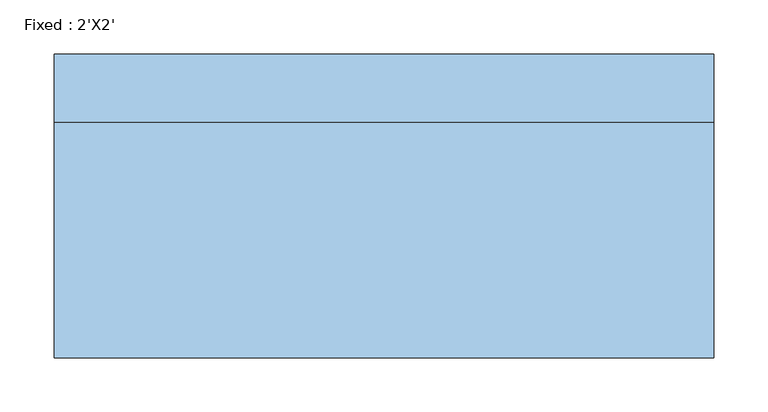
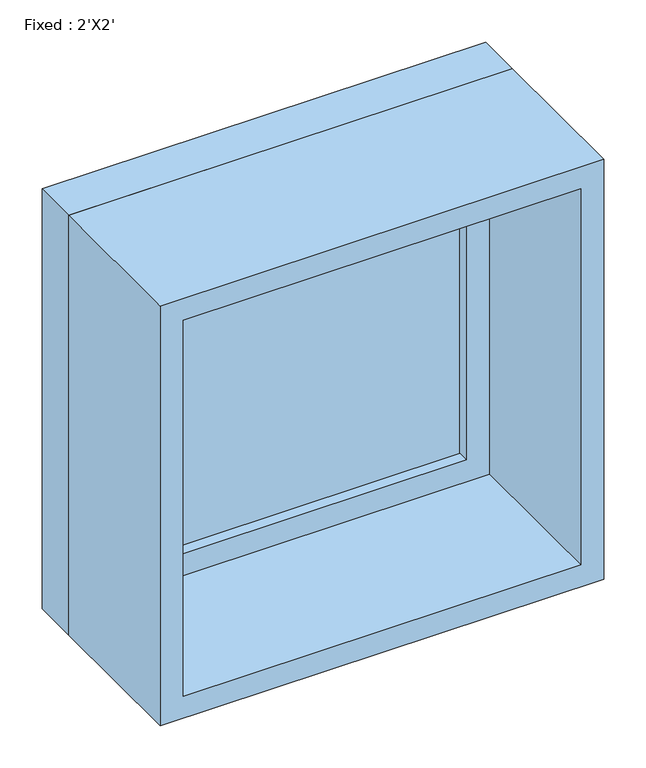
"""IFC4 building model written with IfcOpenShell, lengths in millimetres: window geometry, Fixed : 2'X2'."""

from ifc_helpers import new_model, si_unit, frame, origin, place, context, project, spatial, polyline, outline, extrude, source, transform, mapped, element, save


def fixed_2_x2_ad5176ef(model_context):
    return source(origin(), model_context, "Body", "SweptSolid", [
        extrude(outline(polyline([(203.2, 92.775), (-279.4, 92.775), (-279.4, 105.475), (203.2, 105.475), (203.2, 92.775)])), frame((0.0, 0.0, 977.9), z_axis=(0.0, 0.0, 1.0), x_axis=(1.0, 0.0, 0.0)), (0.0, 0.0, 1.0), 482.6),
        extrude(outline(polyline([(1504.95, -323.85), (933.45, -323.85), (933.45, 247.65), (1504.95, 247.65), (1504.95, -323.85)]), holes=[polyline([(1460.5, -279.4), (1460.5, 203.2), (977.9, 203.2), (977.9, -279.4), (1460.5, -279.4)])]), frame((0.0, 76.9, 0.0), z_axis=(0.0, 1.0, 0.0), x_axis=(0.0, 0.0, 1.0)), (0.0, 0.0, 1.0), 44.45),
        extrude(outline(polyline([(1524.0, -342.9), (914.4, -342.9), (914.4, 266.7), (1524.0, 266.7), (1524.0, -342.9)]), holes=[polyline([(1492.25, -311.15), (1492.25, 234.95), (946.15, 234.95), (946.15, -311.15), (1492.25, -311.15)])]), frame((0.0, -140.4, 0.0), z_axis=(0.0, 1.0, 0.0), x_axis=(0.0, 0.0, 1.0)), (0.0, 0.0, 1.0), 217.3),
        extrude(outline(polyline([(1524.0, 266.7), (1524.0, -342.9), (914.4, -342.9), (914.4, 266.7), (1524.0, 266.7)]), holes=[polyline([(1504.95, 247.65), (933.45, 247.65), (933.45, -323.85), (1504.95, -323.85), (1504.95, 247.65)])]), frame((0.0, 76.9, 0.0), z_axis=(0.0, 1.0, 0.0), x_axis=(0.0, 0.0, 1.0)), (0.0, 0.0, 1.0), 63.5),
    ])


if __name__ == "__main__":
    model = new_model("IFC4")
    model_context = context("Model", 3, world=origin())
    ifc_project = project(units=[si_unit("LENGTHUNIT", "METRE", prefix="MILLI")], contexts=[model_context])
    site = spatial("IfcSite", under=ifc_project)
    building = spatial("IfcBuilding", under=site)
    placement = place(None, origin())
    fixed_2_x2_shape = fixed_2_x2_ad5176ef(model_context)
    element("IfcWindow", 1, ObjectType="Fixed : 2'X2'", at=placement, inside=building, context=model_context, shape_type="MappedRepresentation", body=[
        mapped(fixed_2_x2_shape, transform((0.0, 0.0, 0.0), x_axis=(1.0, 0.0, 0.0), y_axis=(0.0, 1.0, 0.0), z_axis=(0.0, 0.0, 1.0))),
    ])
    save(model, "model.ifc")

# Revit data of these elements
# Type "Fixed : 2'X2'"
#   Type Mark = "11"
#   Assembly Code = "B2020100"
#   Height = 2' - 0"
#   Default Sill Height = 3' - 0"
#   Width = 2' - 0"
#   Window Inset = 0' - 0 3/4"
#   Glass Pane Material = Glass
#   Sash Material = Sash
#   Wall Closure = (empty or 0)
# Element 1 (IfcWindow, "Fixed : 2'X2'")
#   Materials on its faces: "Sash", "Glass"
# Materials
#   "Glass": class "Glass", colour RGB 218 227 224, transparency 0.85, Description = "Soda Lime Glass", Cost = 0
#   "Sash": class "Wood", colour RGB 136 99 55, transparency 0
